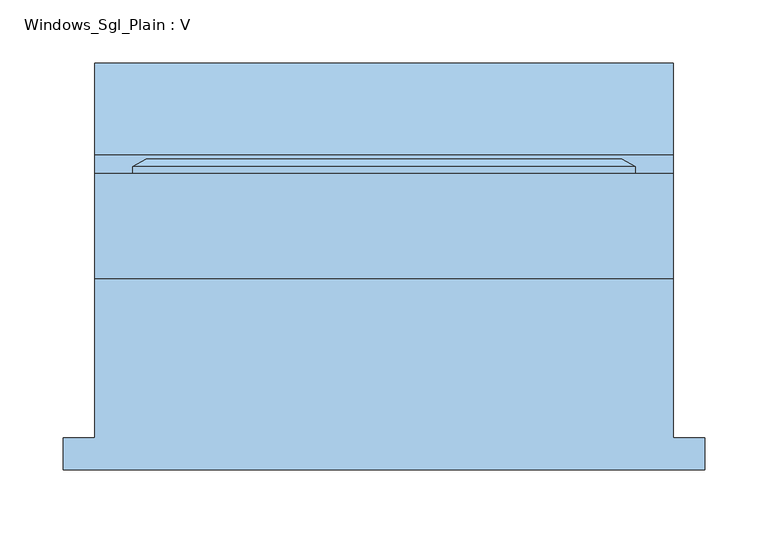
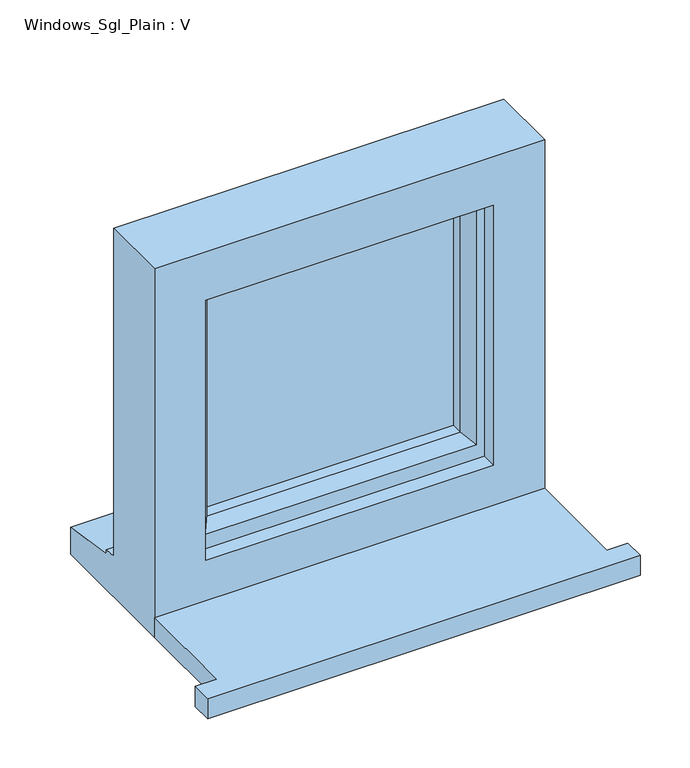
"""IFC4 building model written with IfcOpenShell, lengths in millimetres: window geometry, Windows_Sgl_Plain : V."""

from ifc_helpers import new_model, si_unit, frame, origin, place, context, project, spatial, polyline, outline, extrude, faceted_brep, source, transform, mapped, element, save


def windows_sgl_plain_v_b14593de(model_context):
    return source(origin(), model_context, "Body", "SolidModel", [
        extrude(outline(polyline([(-253.6, -146.0834322), (-253.6, -121.0834322), (-228.6, -121.0834322), (-228.6, 4.9965678), (228.6, 4.9965678), (228.6, -121.0834322), (253.6, -121.0834322), (253.6, -146.0834322), (-253.6, -146.0834322)])), frame((0.0, 0.0, 1652.8), z_axis=(0.0, 0.0, 1.0), x_axis=(1.0, 0.0, 0.0)), (0.0, 0.0, 1.0), 25.0),
        faceted_brep([(-228.6, 4.9965678, 1652.8), (228.6, 4.9965678, 1652.8), (228.6, 4.9965678, 2110.0), (-228.6, 4.9965678, 2110.0), (-168.6, 4.9965678, 2050.0), (168.6, 4.9965678, 2050.0), (168.6, 4.9965678, 1727.8), (-168.6, 4.9965678, 1727.8), (-228.6, 87.9965678, 2110.0), (-228.6, 87.9965678, 1703.8), (-228.6, 102.9965678, 1702.48767), (-228.6, 102.9965678, 1697.5449676), (-228.6, 175.4965678, 1686.6088847), (-228.6, 175.4965678, 1652.8), (228.6, 87.9965678, 2110.0), (228.6, 87.9965678, 1703.8), (-188.6, 87.9965678, 2070.0), (-188.6, 87.9965678, 1715.8), (188.6, 87.9965678, 1715.8), (188.6, 87.9965678, 2070.0), (-188.6, 22.9965678, 2070.0), (-188.6, 22.9965678, 1715.8), (188.6, 22.9965678, 2070.0), (188.6, 22.9965678, 1715.8), (-168.6, 22.9965678, 2050.0), (-168.6, 22.9965678, 1727.8), (168.6, 22.9965678, 1727.8), (168.6, 22.9965678, 2050.0), (228.6, 175.4965678, 1652.8), (228.6, 175.4965678, 1686.6088847), (228.6, 102.9965678, 1697.5449676), (228.6, 102.9965678, 1702.48767)], [[[0, 1, 2, 3], [4, 5, 6, 7]], [[0, 3, 8, 9, 10, 11, 12, 13]], [[9, 8, 14, 15], [16, 17, 18, 19]], [[17, 16, 20, 21]], [[20, 22, 23, 21], [24, 25, 26, 27]], [[24, 4, 7, 25]], [[3, 2, 14, 8]], [[16, 19, 22, 20]], [[5, 4, 24, 27]], [[15, 14, 2, 1, 28, 29, 30, 31]], [[19, 18, 23, 22]], [[5, 27, 26, 6]], [[28, 1, 0, 13]], [[29, 28, 13, 12]], [[30, 29, 12, 11]], [[31, 30, 11, 10]], [[15, 31, 10, 9]], [[21, 23, 18, 17]], [[7, 6, 26, 25]]]),
        extrude(outline(polyline([(158.6, 51.9965678), (-158.6, 51.9965678), (-158.6, 75.9965678), (158.6, 75.9965678), (158.6, 51.9965678)])), frame((0.0, 0.0, 1745.8), z_axis=(0.0, 0.0, 1.0), x_axis=(1.0, 0.0, 0.0)), (0.0, 0.0, 1.0), 294.2),
        faceted_brep([(-198.6, 87.9965678, 2080.0), (-198.6, 93.7700705, 2080.0), (-198.6, 93.7700705, 1705.8), (-198.6, 87.9965678, 1705.8), (-188.6, 22.9965678, 2070.0), (-188.6, 87.9965678, 2070.0), (-188.6, 87.9965678, 1715.8), (-188.6, 22.9965678, 1715.8), (-148.6, 37.4894677, 2030.0), (-158.7480377, 22.9965678, 2040.1480377), (-158.7480377, 22.9965678, 1745.6519623), (-148.6, 37.4894677, 1755.8), (-148.6, 51.9965678, 2030.0), (-148.6, 51.9965678, 1755.8), (-158.6, 75.9965678, 2040.0), (-158.6, 51.9965678, 2040.0), (-158.6, 51.9965678, 1745.8), (-158.6, 75.9965678, 1745.8), (-148.6, 93.7700705, 2030.0), (-148.6, 75.9965678, 2030.0), (-148.6, 75.9965678, 1755.8), (-148.6, 93.7700705, 1755.8), (-166.0457548, 99.5435732, 2047.4457548), (-166.0457548, 99.5435732, 1738.3542452), (-187.8153903, 99.5435732, 2069.2153903), (-187.8153903, 99.5435732, 1716.5846097), (198.6, 93.7700705, 1705.8), (198.6, 87.9965678, 1705.8), (188.6, 87.9965678, 1715.8), (188.6, 22.9965678, 1715.8), (158.7480377, 22.9965678, 1745.6519623), (148.6, 37.4894677, 1755.8), (148.6, 51.9965678, 1755.8), (158.6, 51.9965678, 1745.8), (158.6, 75.9965678, 1745.8), (148.6, 75.9965678, 1755.8), (148.6, 93.7700705, 1755.8), (166.0457548, 99.5435732, 1738.3542452), (187.8153903, 99.5435732, 1716.5846097), (198.6, 93.7700705, 2080.0), (198.6, 87.9965678, 2080.0), (188.6, 87.9965678, 2070.0), (188.6, 22.9965678, 2070.0), (158.7480377, 22.9965678, 2040.1480377), (148.6, 37.4894677, 2030.0), (148.6, 51.9965678, 2030.0), (158.6, 51.9965678, 2040.0), (158.6, 75.9965678, 2040.0), (148.6, 75.9965678, 2030.0), (148.6, 93.7700705, 2030.0), (166.0457548, 99.5435732, 2047.4457548), (187.8153903, 99.5435732, 2069.2153903)], [[[0, 1, 2, 3]], [[4, 5, 6, 7]], [[8, 9, 10, 11]], [[12, 8, 11, 13]], [[14, 15, 16, 17]], [[18, 19, 20, 21]], [[22, 18, 21, 23]], [[1, 24, 25, 2]], [[3, 2, 26, 27]], [[7, 6, 28, 29]], [[11, 10, 30, 31]], [[13, 11, 31, 32]], [[17, 16, 33, 34]], [[21, 20, 35, 36]], [[23, 21, 36, 37]], [[2, 25, 38, 26]], [[27, 26, 39, 40]], [[29, 28, 41, 42]], [[31, 30, 43, 44]], [[32, 31, 44, 45]], [[34, 33, 46, 47]], [[36, 35, 48, 49]], [[37, 36, 49, 50]], [[26, 38, 51, 39]], [[40, 39, 1, 0]], [[3, 27, 40, 0], [5, 41, 28, 6]], [[42, 41, 5, 4]], [[7, 29, 42, 4], [9, 43, 30, 10]], [[44, 43, 9, 8]], [[45, 44, 8, 12]], [[15, 46, 33, 16], [13, 32, 45, 12]], [[47, 46, 15, 14]], [[17, 34, 47, 14], [19, 48, 35, 20]], [[49, 48, 19, 18]], [[50, 49, 18, 22]], [[24, 51, 38, 25], [23, 37, 50, 22]], [[39, 51, 24, 1]]]),
    ])


if __name__ == "__main__":
    model = new_model("IFC4")
    model_context = context("Model", 3, world=origin())
    ifc_project = project(units=[si_unit("LENGTHUNIT", "METRE", prefix="MILLI")], contexts=[model_context])
    site = spatial("IfcSite", under=ifc_project)
    building = spatial("IfcBuilding", under=site)
    placement = place(None, origin())
    windows_sgl_plain_v_shape = windows_sgl_plain_v_b14593de(model_context)
    element("IfcWindow", 1, ObjectType="Windows_Sgl_Plain : V", at=placement, inside=building, context=model_context, shape_type="MappedRepresentation", body=[
        mapped(windows_sgl_plain_v_shape, transform((0.0, 0.0, 0.0), x_axis=(1.0, 0.0, 0.0), y_axis=(0.0, 1.0, 0.0), z_axis=(0.0, 0.0, 1.0))),
    ])
    save(model, "model.ifc")

# Revit data of these elements
# Type "Windows_Sgl_Plain : V"
#   Type Mark = "66"
#   Operation = "SinglePanel"
#   Construction Type Id = "SGL"
#   Manufacturer = "Revit"
#   Keynote = "L10"
#   Analytic Construction = "Large single-glazed windows"
#   Wrap Layers (Ext) from Ext = 102.5 mm
#   Wrap Layers (Int) from Ext = 177.5 mm
#   Window Board Projection = 25 mm
#   Window Board Extension = 25 mm
#   Visual Light Transmittance = 0.9
#   Solar Heat Gain Coefficient = 0.86
#   Rough Width = 457.2 mm
#   Rough Height = 457.2 mm
#   Height = 457.2 mm
#   Width = 457.2 mm
#   Heat Transfer Coefficient (U) = 5.5617 W/(m²·K)
#   Glazing Thickness = 24 mm
#   FrameOffset - External = 50 mm
#   Frame Depth = 65 mm
#   Default Head Height = 2110 mm
#   Cill Depth = 87.5 mm
#   Cavity Closer Width = 50 mm
#   Cavity Closer Offset from Ext = 102.5 mm
#   Cavity Closer Depth = 85 mm
#   Vis - Cavity Closers = yes
#   Define Thermal Properties by = 1
#   Material Trim = Window Frame
#   Material Glass = Glass
#   Material Frame = Window Frame
#   Wall Closure = (empty or 0)
# Element 1 (IfcWindow, "Windows_Sgl_Plain : V")
#   Materials on its faces: "Window Frame", "Glass"
# Materials
#   "Window Frame": colour RGB 249 249 249, transparency 0, Keynote = "L10", Cost = 0
#   "Glass": class "Glass", colour RGB 0 128 192, transparency 0.9, Description = "Soda Lime Glass", Cost = 0
